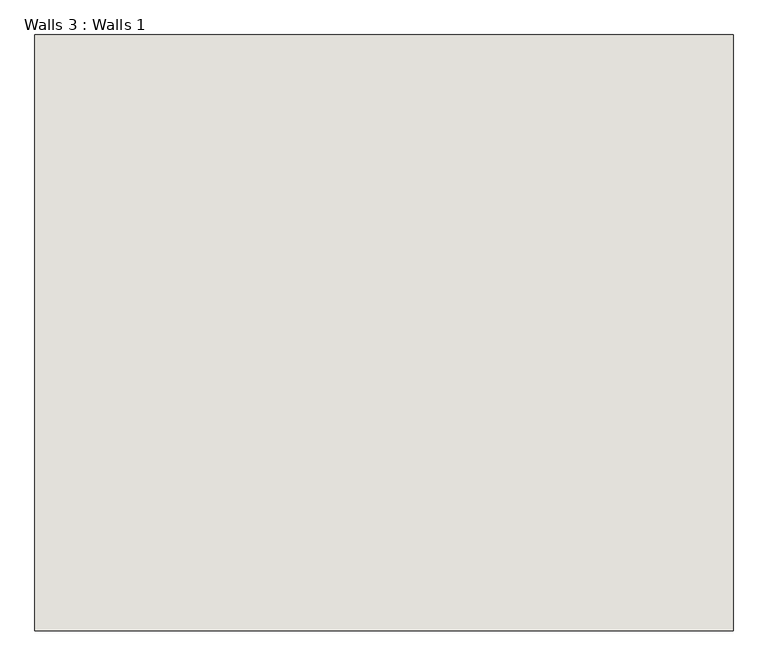
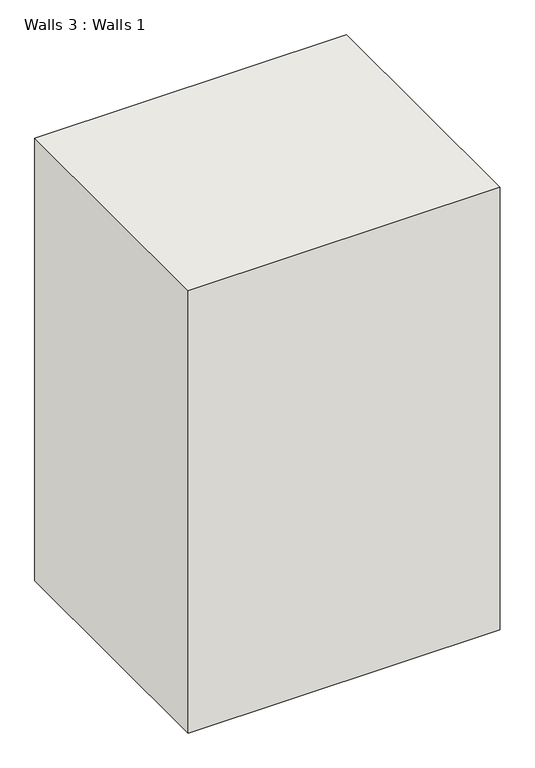
"""IFC4 building model written with IfcOpenShell, lengths in millimetres: wall geometry, Walls 3 : Walls 1."""

from ifc_helpers import new_model, si_unit, frame, origin, place, context, project, spatial, polyline, outline, extrude, source, transform, mapped, element, save


def walls_3_walls_1_4af12cd7(model_context):
    return source(origin(), model_context, "Body", "SweptSolid", [
        extrude(outline(polyline([(-13671.3981295, 1883.8318931), (-14687.3981295, 1883.8318931), (-14687.3981295, 2750.673096), (-13671.3981295, 2750.673096), (-13671.3981295, 1883.8318931)])), frame((0.0, 0.0, 6893.3023612), z_axis=(0.0, 0.0, 1.0), x_axis=(1.0, 0.0, 0.0)), (0.0, 0.0, 1.0), 1524.0),
    ])


if __name__ == "__main__":
    model = new_model("IFC4")
    model_context = context("Model", 3, world=origin())
    ifc_project = project(units=[si_unit("LENGTHUNIT", "METRE", prefix="MILLI")], contexts=[model_context])
    site = spatial("IfcSite", under=ifc_project)
    building = spatial("IfcBuilding", under=site)
    placement = place(None, origin())
    walls_3_walls_1_shape = walls_3_walls_1_4af12cd7(model_context)
    element("IfcWall", 1, ObjectType="Walls 3 : Walls 1", at=placement, inside=building, context=model_context, shape_type="MappedRepresentation", body=[
        mapped(walls_3_walls_1_shape, transform((0.0, 0.0, 0.0), x_axis=(1.0, 0.0, 0.0), y_axis=(0.0, 1.0, 0.0), z_axis=(0.0, 0.0, 1.0))),
    ])
    save(model, "model.ifc")

# Revit data of these elements
# Element 1 (IfcWall, "Walls 3 : Walls 1")
#   Materials on its faces: "Default Wall"
# Materials
#   "Default Wall": colour RGB 128 128 128, transparency 0
